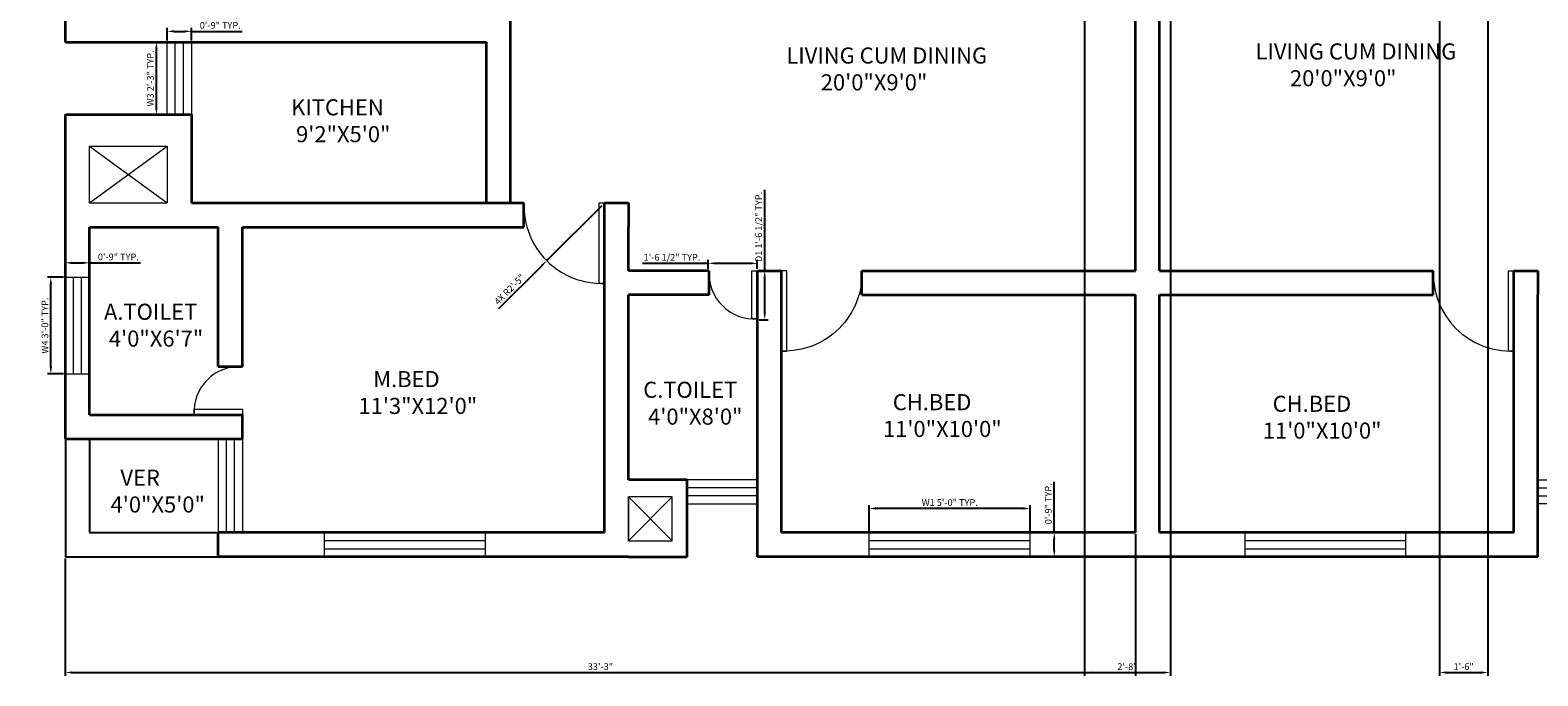
# Model space of a CAD drawing. Units: inches. Extents: x 3941 to 4852, y 2755 to 3388.
# Tile 1 of 5: x 3975 to 4537, y 2755 to 2996. Entities that reach past the tile are written whole.
import ezdxf

# ---------------------------------------------------------------- set-up
doc = ezdxf.new("R2010")
doc.units = ezdxf.units.IN
for name, color, linetype, lineweight in [('A-ANNO-DIMS', 2, 'Continuous', 18), ('A-AREA-IDEN', 7, 'Continuous', 18), ('A-DOOR', 2, 'Continuous', 18), ('A-FLOR-OPEN', 7, 'Continuous', 18), ('A-GLAZ', 5, 'Continuous', 18), ('A-WALL', 7, 'Continuous', 35), ('A-WALL-PRPT', 6, 'Continuous', 25)]:
    doc.layers.add(name, color=color, linetype=linetype, lineweight=lineweight)
doc.styles.get("Standard").update_dxf_attribs({"font": 'arial.ttf'})
doc.dimstyles.new('ISO-25', dxfattribs={"dimtxt": 2.5, "dimasz": 2.5, "dimexe": 1.25, "dimexo": 0.625, "dimtad": 1, "dimlunit": 3, "dimtxsty": 'Standard', "dimcen": 2.5, "dimadec": 0, "dimazin": 0, "dimtfac": 1, "dimtmove": 0, "dimatfit": 3, "dimfxl": 1, "dimarcsym": 0})

# ---------------------------------------------------------------- blocks, each defined once
blk = doc.blocks.new('WINDOW-60IN')
for p, q in [((0, 60), (9, 60)), ((0, 60), (0, 0)), ((3, 60), (3, 0)), ((6, 60), (6, 0)), ((9, 0), (9, 60)), ((0, 0), (9, 0))]:
    blk.add_line(p, q)
blk = doc.blocks.new('WINDOW-27IN')
for p, q in [((0, 0), (0, 27)), ((0, 27), (9, 27)), ((3, 0), (3, 27)), ((6, 0), (6, 27)), ((9, 27), (9, 0)), ((9, 0), (0, 0))]:
    blk.add_line(p, q)
blk = doc.blocks.new('WINDOW-36IN')
for p, q in [((0, 36), (9, 36)), ((0, 36), (0, 0)), ((3, 0), (3, 36)), ((6, 0), (6, 36)), ((9, 0), (9, 36)), ((0, 0), (9, 0))]:
    blk.add_line(p, q)
blk = doc.blocks.new('VERANDA-GLAZING-35IN')
for p, q in [((0, 35), (0, 0)), ((0, 35), (9, 35)), ((3, 35), (3, 0)), ((6, 35), (6, 0)), ((9, 35), (9, 0)), ((9, 35), (9, 0)), ((9, 0), (0, 0))]:
    blk.add_line(p, q)
blk = doc.blocks.new('DOOR-SWING-18IN')
for p, q in [((0.03, 0), (0.03, 2)), ((0.03, 2), (18.03, 2)), ((18.03, 0), (0.03, 0)), ((18.03, 2), (18.03, 0))]:
    blk.add_line(p, q)
blk.add_arc((17.03, 1), 17.03, 86.6335, 183.3665)
blk = doc.blocks.new('DOOR-SWING-30IN')
for p, q in [((0, 30.02), (30, 30.02)), ((0, 28.02), (0, 30.02)), ((30, 30.02), (30, 28.02)), ((30, 28.02), (0, 28.02))]:
    blk.add_line(p, q)
blk.add_arc((1, 29.02), 29.02, 268.0251, 1.9749)
blk = doc.blocks.new('*D11')
at = {"layer": 'A-ANNO-DIMS', "color": 0, "lineweight": -2, "transparency": 16777216}
for p, q in [((4249, 2906.49), (4249, 2936.62)), ((4246.88, 2906.49), (4250.25, 2906.49)), ((4249, 2890.71), (4249, 2903.99)), ((4246.88, 2888.21), (4250.25, 2888.21))]:
    blk.add_line(p, q, dxfattribs=at)
at = {"layer": 'A-ANNO-DIMS', "color": 0, "transparency": 16777216}
for points in [[(4248.58, 2903.99), (4249.41, 2903.99), (4249, 2906.49)], [(4248.58, 2890.71), (4249.41, 2890.71), (4249, 2888.21)]]:
    blk.add_solid(points, dxfattribs=at)
at = {"layer": 'Defpoints', "color": 0, "transparency": 16777216}
for p in [(4246.25, 2906.49), (4249, 2906.49), (4246.25, 2888.21)]:
    blk.add_point(p, dxfattribs=at)
at = {"layer": 'A-ANNO-DIMS', "color": 0, "transparency": 16777216, "insert": (4247.08, 2922.8), "char_height": 2.5, "attachment_point": 5, "rotation": 90}
blk.add_mtext('D1 1\'-6 1/2" TYP.', dxfattribs=at)
blk = doc.blocks.new('*D12')
at = {"layer": 'A-ANNO-DIMS', "color": 0, "lineweight": -2, "transparency": 16777216}
for p, q in [((4227.97, 2909.23), (4203.39, 2909.23)), ((4227.97, 2907.12), (4227.97, 2910.48)), ((4243.75, 2909.23), (4230.47, 2909.23)), ((4246.25, 2907.12), (4246.25, 2910.48))]:
    blk.add_line(p, q, dxfattribs=at)
at = {"layer": 'A-ANNO-DIMS', "color": 0, "transparency": 16777216}
for points in [[(4230.47, 2909.65), (4230.47, 2908.82), (4227.97, 2909.23)], [(4243.75, 2909.65), (4243.75, 2908.82), (4246.25, 2909.23)]]:
    blk.add_solid(points, dxfattribs=at)
at = {"layer": 'Defpoints', "color": 0, "transparency": 16777216}
for p in [(4227.97, 2909.23), (4227.97, 2906.49), (4246.25, 2906.49)]:
    blk.add_point(p, dxfattribs=at)
at = {"layer": 'A-ANNO-DIMS', "color": 0, "transparency": 16777216, "insert": (4214.43, 2911.15), "char_height": 2.5, "attachment_point": 5}
blk.add_mtext('1\'-6 1/2" TYP.', dxfattribs=at)
blk = doc.blocks.new('*D15')
at = {"layer": 'A-ANNO-DIMS', "color": 0, "lineweight": -2, "transparency": 16777216}
for p, q in [((4287.96, 2809.38), (4287.96, 2819)), ((4345.46, 2817.75), (4290.46, 2817.75)), ((4347.96, 2809.38), (4347.96, 2819))]:
    blk.add_line(p, q, dxfattribs=at)
at = {"layer": 'A-ANNO-DIMS', "color": 0, "transparency": 16777216}
for points in [[(4290.46, 2818.17), (4290.46, 2817.34), (4287.96, 2817.75)], [(4345.46, 2818.17), (4345.46, 2817.34), (4347.96, 2817.75)]]:
    blk.add_solid(points, dxfattribs=at)
at = {"layer": 'Defpoints', "color": 0, "transparency": 16777216}
for p in [(4287.96, 2817.75), (4287.96, 2808.75), (4347.96, 2808.75)]:
    blk.add_point(p, dxfattribs=at)
at = {"layer": 'A-ANNO-DIMS', "color": 0, "transparency": 16777216, "insert": (4317.96, 2819.66), "char_height": 2.5, "attachment_point": 5}
blk.add_mtext('W1 5\'-0" TYP.', dxfattribs=at)
blk = doc.blocks.new('*D16')
at = {"layer": 'A-ANNO-DIMS', "color": 0, "lineweight": -2, "transparency": 16777216}
for p, q in [((4356.96, 2808.75), (4356.96, 2827.74)), ((4348.58, 2808.75), (4358.21, 2808.75)), ((4356.96, 2802.25), (4356.96, 2806.25)), ((4348.58, 2799.75), (4358.21, 2799.75))]:
    blk.add_line(p, q, dxfattribs=at)
at = {"layer": 'A-ANNO-DIMS', "color": 0, "transparency": 16777216}
for points in [[(4356.54, 2806.25), (4357.38, 2806.25), (4356.96, 2808.75)], [(4356.54, 2802.25), (4357.38, 2802.25), (4356.96, 2799.75)]]:
    blk.add_solid(points, dxfattribs=at)
at = {"layer": 'Defpoints', "color": 0, "transparency": 16777216}
for p in [(4347.96, 2808.75), (4356.96, 2808.75), (4347.96, 2799.75)]:
    blk.add_point(p, dxfattribs=at)
at = {"layer": 'A-ANNO-DIMS', "color": 0, "transparency": 16777216, "insert": (4355.06, 2819.5), "char_height": 2.5, "attachment_point": 5, "rotation": 90}
blk.add_mtext('0\'-9" TYP.', dxfattribs=at)
blk = doc.blocks.new('*D19')
at = {"layer": 'A-ANNO-DIMS', "color": 0, "lineweight": -2, "transparency": 16777216}
for p, q in [((4025.63, 2991.75), (4020.95, 2991.75)), ((4022.2, 2967.25), (4022.2, 2989.25)), ((4025.63, 2964.75), (4020.95, 2964.75))]:
    blk.add_line(p, q, dxfattribs=at)
at = {"layer": 'A-ANNO-DIMS', "color": 0, "transparency": 16777216}
for points in [[(4021.79, 2989.25), (4022.62, 2989.25), (4022.2, 2991.75)], [(4021.79, 2967.25), (4022.62, 2967.25), (4022.2, 2964.75)]]:
    blk.add_solid(points, dxfattribs=at)
at = {"layer": 'Defpoints', "color": 0, "transparency": 16777216}
for p in [(4022.2, 2991.75), (4026.25, 2991.75), (4026.25, 2964.75)]:
    blk.add_point(p, dxfattribs=at)
at = {"layer": 'A-ANNO-DIMS', "color": 0, "transparency": 16777216, "insert": (4020.3, 2978.25), "char_height": 2.5, "attachment_point": 5, "rotation": 90}
blk.add_mtext('W3 2\'-3" TYP.', dxfattribs=at)
blk = doc.blocks.new('*D20')
at = {"layer": 'A-ANNO-DIMS', "color": 0, "lineweight": -2, "transparency": 16777216}
for p, q in [((4026.25, 2992.38), (4026.25, 2997.05)), ((4035.25, 2992.38), (4035.25, 2997.05)), ((4028.75, 2995.8), (4032.75, 2995.8)), ((4035.25, 2995.8), (4054.24, 2995.8))]:
    blk.add_line(p, q, dxfattribs=at)
at = {"layer": 'A-ANNO-DIMS', "color": 0, "transparency": 16777216}
for points in [[(4028.75, 2996.22), (4028.75, 2995.39), (4026.25, 2995.8)], [(4032.75, 2996.22), (4032.75, 2995.39), (4035.25, 2995.8)]]:
    blk.add_solid(points, dxfattribs=at)
at = {"layer": 'Defpoints', "color": 0, "transparency": 16777216}
for p in [(4026.25, 2991.75), (4035.25, 2995.8), (4035.25, 2991.75)]:
    blk.add_point(p, dxfattribs=at)
at = {"layer": 'A-ANNO-DIMS', "color": 0, "transparency": 16777216, "insert": (4046, 2997.71), "char_height": 2.5, "attachment_point": 5}
blk.add_mtext('0\'-9" TYP.', dxfattribs=at)
blk = doc.blocks.new('*D21')
at = {"layer": 'A-ANNO-DIMS', "color": 0, "lineweight": -2, "transparency": 16777216}
for p, q in [((3987.63, 2904.01), (3981.6, 2904.01)), ((3982.85, 2870.51), (3982.85, 2901.51)), ((3987.63, 2868.01), (3981.6, 2868.01))]:
    blk.add_line(p, q, dxfattribs=at)
at = {"layer": 'A-ANNO-DIMS', "color": 0, "transparency": 16777216}
for points in [[(3982.44, 2901.51), (3983.27, 2901.51), (3982.85, 2904.01)], [(3982.44, 2870.51), (3983.27, 2870.51), (3982.85, 2868.01)]]:
    blk.add_solid(points, dxfattribs=at)
at = {"layer": 'Defpoints', "color": 0, "transparency": 16777216}
for p in [(3982.85, 2904.01), (3988.25, 2904.01), (3988.25, 2868.01)]:
    blk.add_point(p, dxfattribs=at)
at = {"layer": 'A-ANNO-DIMS', "color": 0, "transparency": 16777216, "insert": (3980.95, 2886.01), "char_height": 2.5, "attachment_point": 5, "rotation": 90}
blk.add_mtext('W4 3\'-0" TYP.', dxfattribs=at)
blk = doc.blocks.new('*D22')
at = {"layer": 'A-ANNO-DIMS', "color": 0, "lineweight": -2, "transparency": 16777216}
for p, q in [((3988.25, 2904.63), (3988.25, 2910.66)), ((3990.75, 2909.41), (3994.75, 2909.41)), ((3997.25, 2904.63), (3997.25, 2910.66)), ((3997.25, 2909.41), (4016.24, 2909.41))]:
    blk.add_line(p, q, dxfattribs=at)
at = {"layer": 'A-ANNO-DIMS', "color": 0, "transparency": 16777216}
for points in [[(3990.75, 2909.83), (3990.75, 2908.99), (3988.25, 2909.41)], [(3994.75, 2909.83), (3994.75, 2908.99), (3997.25, 2909.41)]]:
    blk.add_solid(points, dxfattribs=at)
at = {"layer": 'Defpoints', "color": 0, "transparency": 16777216}
for p in [(3997.25, 2909.41), (3988.25, 2904.01), (3997.25, 2904.01)]:
    blk.add_point(p, dxfattribs=at)
at = {"layer": 'A-ANNO-DIMS', "color": 0, "transparency": 16777216, "insert": (4008, 2911.31), "char_height": 2.5, "attachment_point": 5}
blk.add_mtext('0\'-9" TYP.', dxfattribs=at)
blk = doc.blocks.new('*D27')
at = {"layer": 'A-ANNO-DIMS', "color": 0, "lineweight": -2, "transparency": 16777216}
for p, q in [((4368.25, 3318.13), (4368.25, 2755.29)), ((4400.25, 3318.13), (4400.25, 2755.29)), ((4370.75, 2756.54), (4397.75, 2756.54))]:
    blk.add_line(p, q, dxfattribs=at)
at = {"layer": 'A-ANNO-DIMS', "color": 0, "transparency": 16777216}
for points in [[(4370.75, 2756.96), (4370.75, 2756.13), (4368.25, 2756.54)], [(4397.75, 2756.96), (4397.75, 2756.13), (4400.25, 2756.54)]]:
    blk.add_solid(points, dxfattribs=at)
at = {"layer": 'Defpoints', "color": 0, "transparency": 16777216}
for p in [(4368.25, 3318.75), (4400.25, 3318.75), (4400.25, 2756.54)]:
    blk.add_point(p, dxfattribs=at)
at = {"layer": 'A-ANNO-DIMS', "color": 0, "transparency": 16777216, "insert": (4384.25, 2758.44), "char_height": 2.5, "attachment_point": 5}
blk.add_mtext('2\'-8"', dxfattribs=at)
blk = doc.blocks.new('*D28')
at = {"layer": 'A-ANNO-DIMS', "color": 0, "lineweight": -2, "transparency": 16777216}
for p, q in [((4387.25, 2808.13), (4387.25, 2755.29)), ((3988.25, 2799.13), (3988.25, 2755.29)), ((3990.75, 2756.54), (4384.75, 2756.54))]:
    blk.add_line(p, q, dxfattribs=at)
at = {"layer": 'A-ANNO-DIMS', "color": 0, "transparency": 16777216}
for points in [[(3990.75, 2756.96), (3990.75, 2756.13), (3988.25, 2756.54)], [(4384.75, 2756.96), (4384.75, 2756.13), (4387.25, 2756.54)]]:
    blk.add_solid(points, dxfattribs=at)
at = {"layer": 'Defpoints', "color": 0, "transparency": 16777216}
for p in [(4387.25, 2808.75), (3988.25, 2799.75), (4387.25, 2756.54)]:
    blk.add_point(p, dxfattribs=at)
at = {"layer": 'A-ANNO-DIMS', "color": 0, "transparency": 16777216, "insert": (4187.75, 2758.44), "char_height": 2.5, "attachment_point": 5}
blk.add_mtext('33\'-3"', dxfattribs=at)
blk = doc.blocks.new('*D38')
at = {"layer": 'A-ANNO-DIMS', "color": 0, "lineweight": -2, "transparency": 16777216}
for p, q in [((4500.59, 3318.13), (4500.59, 2755.29)), ((4518.59, 3318.13), (4518.59, 2755.29)), ((4503.09, 2756.54), (4516.09, 2756.54))]:
    blk.add_line(p, q, dxfattribs=at)
at = {"layer": 'A-ANNO-DIMS', "color": 0, "transparency": 16777216}
for points in [[(4503.09, 2756.96), (4503.09, 2756.13), (4500.59, 2756.54)], [(4516.09, 2756.96), (4516.09, 2756.13), (4518.59, 2756.54)]]:
    blk.add_solid(points, dxfattribs=at)
at = {"layer": 'Defpoints', "color": 0, "transparency": 16777216}
for p in [(4500.59, 3318.75), (4518.59, 3318.75), (4518.59, 2756.54)]:
    blk.add_point(p, dxfattribs=at)
at = {"layer": 'A-ANNO-DIMS', "color": 0, "transparency": 16777216, "insert": (4509.59, 2758.44), "char_height": 2.5, "attachment_point": 5}
blk.add_mtext('1\'-6"', dxfattribs=at)
blk = doc.blocks.new('*D46')
at = {"layer": 'A-ANNO-DIMS', "color": 0, "lineweight": -2, "transparency": 16777216}
for p, q in [((4188.25, 2930.75), (4167.74, 2910.24)), ((4149.85, 2892.35), (4165.97, 2908.47))]:
    blk.add_line(p, q, dxfattribs=at)
at = {"layer": 'A-ANNO-DIMS', "color": 0, "transparency": 16777216}
blk.add_solid([(4165.67, 2908.76), (4166.26, 2908.17), (4167.74, 2910.24)], dxfattribs=at)
at = {"layer": 'Defpoints', "color": 0, "transparency": 16777216}
for p in [(4188.25, 2930.75), (4167.74, 2910.24)]:
    blk.add_point(p, dxfattribs=at)
at = {"layer": 'A-ANNO-DIMS', "color": 0, "transparency": 16777216, "insert": (4154.08, 2899.27), "char_height": 2.5, "attachment_point": 5, "rotation": 44.9996}
blk.add_mtext('4X R2\'-5"', dxfattribs=at)

msp = doc.modelspace()

# ---------------------------------------------------------------- linework, layer by layer
at = {"layer": 'A-FLOR-OPEN'}
for p, q in [((3997.254, 2931.754), (3997.254, 2952.917)), ((3997.254, 2952.917), (4026.254, 2952.917)), ((3997.254, 2931.754), (4026.254, 2952.917)), ((3997.254, 2952.917), (4026.254, 2931.754)), ((4026.254, 2952.917), (4026.254, 2931.754)), ((3997.254, 2931.754), (3997.254, 2948.254)), ((3997.254, 2931.754), (4026.254, 2931.754)), ((4198.254, 2822.116), (4198.254, 2805.703)), ((4214.506, 2822.116), (4198.254, 2822.116)), ((4214.506, 2822.116), (4198.254, 2805.703)), ((4198.254, 2805.703), (4198.254, 2822.116)), ((4198.254, 2822.116), (4214.506, 2805.703)), ((4214.506, 2805.703), (4214.506, 2822.116)), ((4198.254, 2805.703), (4214.506, 2805.703))]:
    msp.add_line(p, q, dxfattribs=at)
at = {"layer": 'A-GLAZ'}
for p, q in [((4246.254, 2828.492), (4220.048, 2828.492)), ((4220.048, 2828.492), (4220.048, 2819.492)), ((4246.254, 2819.492), (4246.254, 2828.492)), ((4246.254, 2825.492), (4220.048, 2825.492)), ((4246.254, 2822.492), (4220.048, 2822.492)), ((4220.048, 2819.492), (4246.254, 2819.492)), ((4428.082, 2808.754), (4428.082, 2808.754))]:
    msp.add_line(p, q, dxfattribs=at)
at = {"layer": 'A-WALL'}
for p, q in [((3988.254, 2991.754), (3988.254, 3129.754)), ((4387.254, 2906.492), (4387.254, 3080.521)), ((4396.254, 2906.492), (4396.254, 3080.521)), ((4154.254, 2931.754), (4154.254, 3028.754)), ((3988.254, 2991.754), (4145.254, 2991.754)), ((4145.254, 2931.754), (4145.254, 2991.754)), ((3988.254, 2922.754), (3988.254, 2964.754)), ((3988.254, 2964.754), (4035.254, 2964.754)), ((3988.254, 2843.754), (3988.254, 2964.754)), ((4035.254, 2964.754), (4035.254, 2931.754)), ((4035.254, 2931.754), (4154.254, 2931.754)), ((4154.254, 2931.754), (4159.254, 2931.754)), ((4159.254, 2922.754), (4159.254, 2931.754)), ((4189.254, 2808.754), (4189.254, 2931.754)), ((4189.254, 2931.754), (4198.254, 2931.754)), ((4198.254, 2931.754), (4198.254, 2922.754)), ((3997.254, 2922.754), (4045.254, 2922.754)), ((3997.254, 2852.754), (3997.254, 2922.754)), ((4045.254, 2870.754), (4045.254, 2922.754)), ((4054.254, 2922.754), (4159.254, 2922.754)), ((4054.254, 2870.754), (4054.254, 2922.754)), ((4198.254, 2906.492), (4198.254, 2922.754)), ((4228.254, 2906.492), (4198.254, 2906.492)), ((4228.254, 2897.492), (4228.254, 2906.492)), ((4246.254, 2897.492), (4246.254, 2906.492)), ((4246.254, 2906.492), (4255.254, 2906.492)), ((4255.254, 2808.754), (4255.254, 2906.492)), ((4285.254, 2906.492), (4387.254, 2906.492)), ((4285.254, 2897.492), (4285.254, 2906.492)), ((4396.254, 2906.492), (4498.254, 2906.492)), ((4498.254, 2897.492), (4498.254, 2906.492)), ((4528.254, 2808.754), (4528.254, 2906.492)), ((4528.254, 2906.492), (4537.254, 2906.492)), ((4537.254, 2906.492), (4537.254, 2897.492)), ((4198.254, 2828.492), (4198.254, 2897.492)), ((4228.254, 2897.492), (4198.254, 2897.492)), ((4246.254, 2799.754), (4246.254, 2897.492)), ((4285.254, 2897.492), (4387.254, 2897.492)), ((4387.254, 2808.754), (4387.254, 2897.492)), ((4396.254, 2808.754), (4396.254, 2897.492)), ((4396.254, 2808.754), (4396.254, 2897.492)), ((4396.254, 2897.492), (4498.254, 2897.492)), ((4537.254, 2799.754), (4537.254, 2897.492)), ((4045.254, 2870.754), (4054.254, 2870.754)), ((3997.254, 2852.754), (4054.254, 2852.754)), ((4054.254, 2843.754), (4054.254, 2852.754)), ((3988.254, 2843.754), (4054.254, 2843.754)), ((4220.048, 2828.492), (4198.254, 2828.492)), ((4220.048, 2799.754), (4220.048, 2828.492)), ((4045.254, 2799.754), (4045.254, 2808.754)), ((4189.254, 2808.754), (4045.254, 2808.754)), ((4387.254, 2808.754), (4255.254, 2808.754)), ((4528.254, 2808.754), (4396.254, 2808.754)), ((4198.254, 2799.754), (4045.254, 2799.754)), ((4198.254, 2799.754), (4220.048, 2799.754)), ((4537.254, 2799.754), (4246.254, 2799.754))]:
    msp.add_line(p, q, dxfattribs=at)
at = {"layer": 'A-WALL-PRPT'}
for p, q in [((3988.254, 2843.754), (3988.254, 2799.754)), ((3997.254, 2843.754), (3997.254, 2808.754)), ((3997.254, 2808.754), (4045.254, 2808.754)), ((3988.254, 2799.754), (4045.254, 2799.754))]:
    msp.add_line(p, q, dxfattribs=at)

# ---------------------------------------------------------------- block references
at = {"layer": 'A-DOOR'}
for name, p, rotation in [('DOOR-SWING-30IN', (4159.237, 2931.754), 270.0000000000011), ('DOOR-SWING-18IN', (4246.254, 2888.462), 90.00000000000252), ('DOOR-SWING-30IN', (4498.237, 2906.492), 269.9999999999996)]:
    msp.add_blockref(name, p, dxfattribs=dict(at, rotation=rotation))
at = {"layer": 'A-DOOR', "extrusion": (0, 0, -1), "zscale": -1, "rotation": 270.0000000000027}
msp.add_blockref('DOOR-SWING-30IN', (-4285.27, 2906.492), dxfattribs=at)
at = {"layer": 'A-DOOR'}
msp.add_blockref('DOOR-SWING-18IN', (4036.224, 2852.754), dxfattribs=at)
at = {"layer": 'A-GLAZ'}
for name, p in [('WINDOW-27IN', (4026.254, 2964.754)), ('WINDOW-36IN', (3988.254, 2868.009)), ('VERANDA-GLAZING-35IN', (4045.254, 2808.754))]:
    msp.add_blockref(name, p, dxfattribs=at)
for name, p, rotation in [('WINDOW-27IN', (4537.253, 2828.492), 270.0000000000023), ('WINDOW-60IN', (4144.886, 2799.755), 89.99999999999936), ('WINDOW-60IN', (4347.96, 2799.755), 90), ('WINDOW-60IN', (4488.081, 2799.755), 90)]:
    msp.add_blockref(name, p, dxfattribs=dict(at, rotation=rotation))

# ---------------------------------------------------------------- texts
at = {"layer": 'A-AREA-IDEN', "char_height": 6, "attachment_point": 1}
for s, width, heights, insert in [(' LIVING CUM DINING\\P        20\'0"X9\'0"', 233.06976, [115.113], (4430.171, 2991.306)), (' LIVING CUM DINING\\P        20\'0"X9\'0"', 233.06976, [115.113], (4255.241, 2989.775)), (' KITCHEN\\P  9\'2"X5\'0"', 69.57529, [0], (4070.619, 2970.438)), ('A.TOILET\\P 4\'0"X6\'7"', 69.57529, [0], (4002.661, 2894.154)), ('    M.BED\\P 11\'3"X12\'0"', 69.57529, [0], (4095.715, 2869.024)), (' C.TOILET\\P  4\'0"X8\'0"', 69.57529, [0], (4201.869, 2865.042)), ('   CH.BED\\P 11\'0"X10\'0"', 69.57529, [0], (4291.265, 2860.423)), ('   CH.BED\\P 11\'0"X10\'0"', 69.57529, [0], (4432.879, 2859.816)), ('  VER\\P4\'0"X5\'0"', 69.57529, [0], (4005.117, 2832.24))]:
    msp.add_mtext_dynamic_manual_height_columns(s, width=width, gutter_width=12.5, heights=heights, dxfattribs=dict(at, insert=insert))

# ---------------------------------------------------------------- dimensions: what is measured, and where the dimension line sits
at = {"layer": 'A-ANNO-DIMS'}
for base, p1, p2, picture, middle in [((4400.254, 2756.542), (4368.254, 3318.754), (4400.254, 3318.754), '*D27', (4384.254, 2758.443)), ((4518.593, 2756.542), (4500.593, 3318.754), (4518.593, 3318.754), '*D38', (4509.593, 2758.443)), ((4387.254, 2756.542), (3988.254, 2799.754), (4387.254, 2808.754), '*D28', (4187.754, 2758.444))]:
    dim = msp.add_linear_dim(base=base, p1=p1, p2=p2, dimstyle='ISO-25', override={"dimdec": 1, "dimlfac": 1, "dimrnd": 0, "dimzin": 1, "dimdsep": 46, "dimlunit": 4, "dimfrac": 2}, dxfattribs=at)
    dim.commit()
    dim.dimension.update_dxf_attribs({"geometry": picture, "text_midpoint": middle})
for base, p1, p2, picture, middle in [((4035.254, 2995.804), (4026.254, 2991.754), (4035.254, 2991.754), '*D20', (4045.998, 2997.706)), ((3997.254, 2909.409), (3988.254, 2904.009), (3997.254, 2904.009), '*D22', (4007.998, 2911.31))]:
    dim = msp.add_linear_dim(base=base, p1=p1, p2=p2, text='<> TYP.', dimstyle='ISO-25', override={"dimdec": 1, "dimlfac": 1, "dimrnd": 0, "dimzin": 1, "dimdsep": 46, "dimlunit": 4, "dimfrac": 2}, dxfattribs=at)
    dim.commit()
    dim.dimension.update_dxf_attribs({"geometry": picture, "text_midpoint": middle})
for base, p1, p2, angle, text, picture, middle in [((4022.204, 2991.754), (4026.254, 2964.754), (4026.254, 2991.754), 90, 'W3 <> TYP.', '*D19', (4020.301, 2978.254)), ((4248.996, 2906.492), (4246.254, 2888.206), (4246.254, 2906.492), 90, 'D1 <> TYP.', '*D11', (4247.079, 2922.804)), ((4227.968, 2909.235), (4246.254, 2906.492), (4227.968, 2906.492), 180, '<> TYP.', '*D12', (4214.429, 2911.153)), ((3982.854, 2904.009), (3988.254, 2868.009), (3988.254, 2904.009), 90, 'W4 <> TYP.', '*D21', (3980.951, 2886.009)), ((4356.96, 2808.754), (4347.96, 2799.754), (4347.96, 2808.754), 90, '<> TYP.', '*D16', (4355.058, 2819.499)), ((4287.96, 2817.754), (4347.96, 2808.754), (4287.96, 2808.754), 180, 'W1 <> TYP.', '*D15', (4317.96, 2819.656))]:
    dim = msp.add_linear_dim(base=base, p1=p1, p2=p2, angle=angle, text=text, dimstyle='ISO-25', override={"dimdec": 1, "dimlfac": 1, "dimrnd": 0, "dimzin": 1, "dimdsep": 46, "dimlunit": 4, "dimfrac": 2}, dxfattribs=at)
    dim.commit()
    dim.dimension.update_dxf_attribs({"geometry": picture, "text_midpoint": middle})
dim = msp.add_radius_dim(center=(4188.254, 2930.754), mpoint=(4167.735, 2910.236), text='4X <>', dimstyle='ISO-25', override={"dimdec": 1, "dimlfac": 1, "dimrnd": 0, "dimzin": 1, "dimdsep": 46, "dimlunit": 4, "dimfrac": 2}, dxfattribs=at)
dim.commit()
dim.dimension.update_dxf_attribs({"geometry": '*D46', "text_midpoint": (4155.424, 2897.925), "dimtype": 164})

doc.saveas('drawing.dxf')
